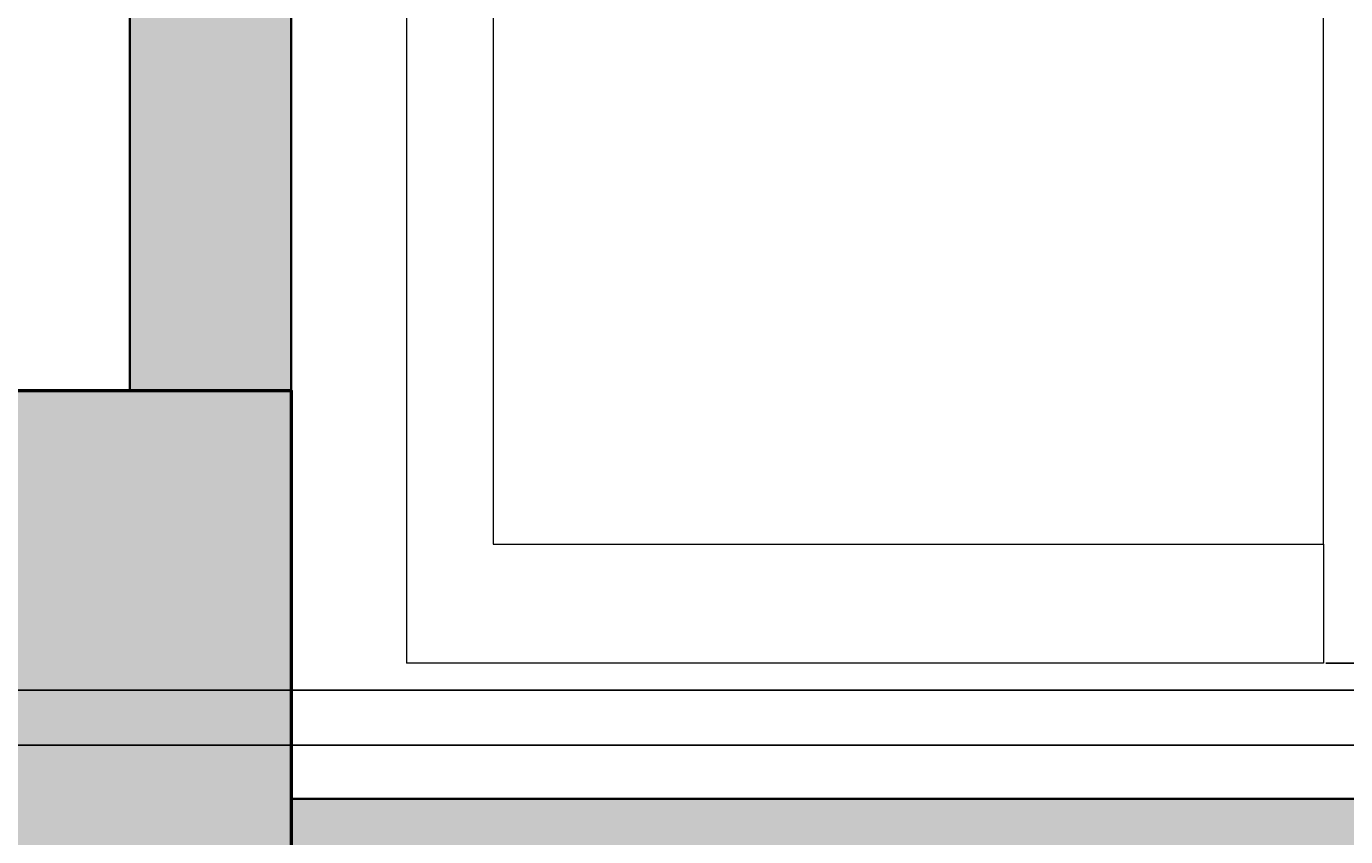
# Model space of a CAD drawing. Units: inches. Extents: x 1998 to 2588, y 1139 to 1977.
# Tile 43 of 134: x 2220 to 2257, y 1592 to 1615. Entities that reach past the tile are written whole.
import ezdxf

# ---------------------------------------------------------------- set-up
doc = ezdxf.new("R2010")
doc.units = ezdxf.units.IN
for name, color, linetype, lineweight in [('A-ANNO-DIMS', 2, 'Continuous', 18), ('A-COLS-PATT', 250, 'Continuous', 13), ('A-WALL-PATT', 252, 'Continuous', 13), ('COLUMN', 10, 'Continuous', 50), ('FUR', 21, 'Continuous', 18), ('WALL', 200, 'Continuous', 35)]:
    doc.layers.add(name, color=color, linetype=linetype, lineweight=lineweight)
doc.styles.get("Standard").update_dxf_attribs({"font": 'arial.ttf'})
doc.dimstyles.get("Standard").update_dxf_attribs({"dimtxt": 0.18, "dimasz": 0.18, "dimexe": 0.18, "dimexo": 0.0625, "dimgap": 0.09, "dimtad": 0, "dimtih": 1, "dimtoh": 1, "dimdec": 4, "dimzin": 0, "dimdsep": 46, "dimtxsty": 'Standard', "dimcen": 0.09, "dimadec": 0, "dimazin": 0, "dimtfac": 1, "dimtdec": 4, "dimtofl": 0, "dimtmove": 0, "dimatfit": 3, "dimfxl": 1, "dimtolj": 1, "dimtzin": 0, "dimarcsym": 0})

# ---------------------------------------------------------------- blocks, each defined once
blk = doc.blocks.new('SOFA-THREE-SEAT')
for p, q in [((71.008, 25.615), (74.336, 25.615)), ((74.336, 25.615), (74.336, 0)), ((0, 0), (74.336, 0))]:
    blk.add_line(p, q)
blk.add_lwpolyline([(3.604, 2.416), (71.008, 2.416), (71.008, 25.615), (3.604, 25.615)], close=True)
blk = doc.blocks.new('*D11')
at = {"layer": 'A-ANNO-DIMS', "color": 0, "lineweight": -2, "transparency": 16777216}
for p, q in [((2256.378, 1671.356), (2267.646, 1671.356)), ((2267.466, 1671.176), (2267.466, 1634.372)), ((2267.466, 1597.201), (2267.466, 1634.005)), ((2256.378, 1597.021), (2267.646, 1597.021))]:
    blk.add_line(p, q, dxfattribs=at)
at = {"layer": 'A-ANNO-DIMS', "color": 0, "transparency": 16777216}
for points in [[(2267.436, 1671.176), (2267.496, 1671.176), (2267.466, 1671.356)], [(2267.436, 1597.201), (2267.496, 1597.201), (2267.466, 1597.021)]]:
    blk.add_solid(points, dxfattribs=at)
at = {"layer": 'Defpoints', "color": 0, "transparency": 16777216}
for p in [(2256.316, 1671.356), (2256.316, 1597.021), (2267.466, 1597.021)]:
    blk.add_point(p, dxfattribs=at)
at = {"layer": 'A-ANNO-DIMS', "color": 0, "transparency": 16777216, "insert": (2267.466, 1634.189), "char_height": 0.18, "attachment_point": 5}
blk.add_mtext('\\A1;SOFA 74 TYP.', dxfattribs=at)
blk = doc.blocks.new('*D30')
at = {"layer": 'A-ANNO-DIMS', "color": 0, "lineweight": -2, "transparency": 16777216}
for p, q in [((2407.91, 1636.732), (1997.843, 1636.732)), ((1998.023, 1636.552), (1998.023, 1615.913)), ((1998.023, 1594.912), (1998.023, 1615.552)), ((2407.91, 1594.732), (1997.843, 1594.732))]:
    blk.add_line(p, q, dxfattribs=at)
at = {"layer": 'A-ANNO-DIMS', "color": 0, "transparency": 16777216}
for points in [[(1997.993, 1636.552), (1998.053, 1636.552), (1998.023, 1636.732)], [(1997.993, 1594.912), (1998.053, 1594.912), (1998.023, 1594.732)]]:
    blk.add_solid(points, dxfattribs=at)
at = {"layer": 'Defpoints', "color": 0, "transparency": 16777216}
for p in [(1998.023, 1636.732), (2407.973, 1636.732), (2407.973, 1594.732)]:
    blk.add_point(p, dxfattribs=at)
at = {"layer": 'A-ANNO-DIMS', "color": 0, "transparency": 16777216, "insert": (1998.023, 1615.732), "char_height": 0.18, "attachment_point": 5}
blk.add_mtext('\\A1;42', dxfattribs=at)
blk = doc.blocks.new('*D34')
at = {"layer": 'A-ANNO-DIMS', "color": 0, "lineweight": -2, "transparency": 16777216}
for p, q in [((2407.91, 1594.732), (1997.843, 1594.732)), ((1998.023, 1594.552), (1998.023, 1558.913)), ((1998.023, 1522.912), (1998.023, 1558.552)), ((2407.91, 1522.732), (1997.843, 1522.732))]:
    blk.add_line(p, q, dxfattribs=at)
at = {"layer": 'A-ANNO-DIMS', "color": 0, "transparency": 16777216}
for points in [[(1997.993, 1594.552), (1998.053, 1594.552), (1998.023, 1594.732)], [(1997.993, 1522.912), (1998.053, 1522.912), (1998.023, 1522.732)]]:
    blk.add_solid(points, dxfattribs=at)
at = {"layer": 'Defpoints', "color": 0, "transparency": 16777216}
for p in [(1998.023, 1594.732), (2407.973, 1594.732), (2407.973, 1522.732)]:
    blk.add_point(p, dxfattribs=at)
at = {"layer": 'A-ANNO-DIMS', "color": 0, "transparency": 16777216, "insert": (1998.023, 1558.732), "char_height": 0.18, "attachment_point": 5}
blk.add_mtext('\\A1;72', dxfattribs=at)
blk = doc.blocks.new('*D39')
at = {"layer": 'A-ANNO-DIMS', "color": 0, "lineweight": -2, "transparency": 16777216}
for p, q in [((2115.035, 1628.742), (2588.309, 1628.742)), ((2588.129, 1628.562), (2588.129, 1612.685)), ((2588.129, 1596.444), (2588.129, 1612.321)), ((2115.035, 1596.264), (2588.309, 1596.264))]:
    blk.add_line(p, q, dxfattribs=at)
at = {"layer": 'A-ANNO-DIMS', "color": 0, "transparency": 16777216}
for points in [[(2588.099, 1628.562), (2588.159, 1628.562), (2588.129, 1628.742)], [(2588.099, 1596.444), (2588.159, 1596.444), (2588.129, 1596.264)]]:
    blk.add_solid(points, dxfattribs=at)
at = {"layer": 'Defpoints', "color": 0, "transparency": 16777216}
for p in [(2114.973, 1628.742), (2588.129, 1628.742), (2114.973, 1596.264)]:
    blk.add_point(p, dxfattribs=at)
at = {"layer": 'A-ANNO-DIMS', "color": 0, "transparency": 16777216, "insert": (2588.129, 1612.503), "char_height": 0.18, "attachment_point": 5}
blk.add_mtext('\\A1;32.48', dxfattribs=at)

msp = doc.modelspace()

# ---------------------------------------------------------------- hatches: boundary and pattern name
at = {"layer": 'A-COLS-PATT'}
h = msp.add_hatch(color=256, dxfattribs=at)
h.dxf.hatch_style = 1
h.paths.add_polyline_path([(2099.4125, 1888.7324), (2087.9729, 1888.7324), (2087.9729, 1868.3278), (2099.4125, 1868.3278)])
h.paths.add_polyline_path([(2234.4125, 1888.7324), (2222.9729, 1888.7324), (2222.9729, 1868.3278), (2234.4125, 1868.3278)])
h.paths.add_polyline_path([(2341.4729, 1886.637), (2330.0332, 1886.637), (2330.0332, 1866.2324), (2341.4729, 1866.2324)])
h.paths.add_polyline_path([(2507.8006, 1882.7324), (2487.396, 1882.7324), (2487.396, 1871.2927), (2507.8006, 1871.2927)])
h.paths.add_polyline_path([(2510.9729, 1766.672), (2490.5682, 1766.672), (2490.5682, 1755.2324), (2510.9729, 1755.2324)])
h.paths.add_polyline_path([(2345.9729, 1759.7324), (2334.5332, 1759.7324), (2334.5332, 1739.3278), (2345.9729, 1739.3278)])
h.paths.add_polyline_path([(2234.4125, 1774.3318), (2222.9729, 1774.3318), (2222.9729, 1753.9272), (2234.4125, 1753.9272)])
h.paths.add_polyline_path([(2099.4125, 1775.637), (2087.9729, 1775.637), (2087.9729, 1755.2324), (2099.4125, 1755.2324)])
h.paths.add_polyline_path([(2098.0956, 1593.7241), (2077.691, 1593.7241), (2077.691, 1582.2845), (2098.0956, 1582.2845)])
h.paths.add_polyline_path([(2227.4729, 1604.637), (2216.0332, 1604.637), (2216.0332, 1584.2324), (2227.4729, 1584.2324)])
h.paths.add_polyline_path([(2345.9729, 1647.5211), (2334.5332, 1647.5211), (2334.5332, 1627.1165), (2345.9729, 1627.1165)])
h.paths.add_polyline_path([(2522.3775, 1641.2324), (2501.9729, 1641.2324), (2501.9729, 1629.7927), (2522.3775, 1629.7927)])
h.paths.add_polyline_path([(2522.3775, 1480.7324), (2501.9729, 1480.7324), (2501.9729, 1469.2927), (2522.3775, 1469.2927)])
h.paths.add_polyline_path([(2345.9729, 1488.5616), (2334.5332, 1488.5616), (2334.5332, 1468.1569), (2345.9729, 1468.1569)])
h.paths.add_polyline_path([(2234.4125, 1486.137), (2227.4729, 1486.137), (2227.4729, 1465.7324), (2234.4125, 1465.7324)])
h.paths.add_polyline_path([(2227.4729, 1486.137), (2222.9729, 1486.137), (2222.9729, 1465.7324), (2227.4729, 1465.7324)])
h.paths.add_polyline_path([(2108.3775, 1470.2324), (2087.9729, 1470.2324), (2087.9729, 1458.7927), (2108.3775, 1458.7927)])
h.paths.add_polyline_path([(2096.9729, 1365.5012), (2087.9729, 1365.5012), (2087.9729, 1345.0966), (2096.9729, 1345.0966)])
h.paths.add_polyline_path([(2087.9729, 1365.5012), (2085.5332, 1365.5012), (2085.5332, 1345.0966), (2087.9729, 1345.0966)])
h.paths.add_polyline_path([(2234.4125, 1285.137), (2222.9729, 1285.137), (2222.9729, 1264.7324), (2234.4125, 1264.7324)])
h.paths.add_polyline_path([(2345.9729, 1285.137), (2334.5332, 1285.137), (2334.5332, 1264.7324), (2345.9729, 1264.7324)])
h.paths.add_polyline_path([(2503.1458, 1240.172), (2482.7412, 1240.172), (2482.7412, 1228.7324), (2503.1458, 1228.7324)])
h.paths.add_polyline_path([(2510.9729, 1369.172), (2490.5682, 1369.172), (2490.5682, 1357.7324), (2510.9729, 1357.7324)])
at = {"layer": 'A-WALL-PATT'}
h = msp.add_hatch(color=256, dxfattribs=at)
h.dxf.hatch_style = 1
h.paths.add_polyline_path([(2222.9729, 1888.7324), (2099.4125, 1888.7324), (2099.4125, 1879.7324), (2222.9729, 1879.7324)])
h.paths.add_polyline_path([(2096.9729, 1868.3278), (2087.9729, 1868.3278), (2087.9729, 1775.637), (2096.9729, 1775.637)])
h.paths.add_polyline_path([(2227.4729, 1868.3278), (2222.9729, 1868.3278), (2222.9729, 1774.3318), (2227.4729, 1774.3318)])
h.paths.add_polyline_path([(2188.3019, 1759.7324), (2138.6074, 1759.7324), (2099.4125, 1759.7324), (2099.4125, 1755.2324), (2176.9729, 1755.2324), (2188.3019, 1755.2324)])
h.paths.add_polyline_path([(2087.9729, 1759.7324), (2059.4729, 1759.7324), (2059.4729, 1702.7324), (2087.9729, 1702.7324), (2087.9729, 1707.2324), (2063.9729, 1707.2324), (2063.9729, 1755.2324), (2087.9729, 1755.2324)])
h.paths.add_polyline_path([(2096.9729, 1755.2324), (2087.9729, 1755.2324), (2087.9729, 1707.2324), (2096.9729, 1707.2324)])
h.paths.add_polyline_path([(2187.0461, 1707.2324), (2105.9729, 1707.2324), (2096.9729, 1707.2324), (2087.9729, 1707.2324), (2087.9729, 1702.7324), (2105.9729, 1702.7324), (2114.9729, 1702.7324), (2187.0461, 1702.7324)])
h.paths.add_polyline_path([(2181.4729, 1719.2028), (2176.9729, 1719.2028), (2176.9729, 1707.2324), (2181.4729, 1707.2324)])
h.paths.add_polyline_path([(2216.0332, 1588.7324), (2114.9729, 1588.7324), (2105.9729, 1588.7324), (2105.9729, 1584.2324), (2216.0332, 1584.2324)])
h.paths.add_polyline_path([(2077.691, 1588.7324), (2061.4729, 1588.7324), (2061.4729, 1584.2324), (2077.691, 1584.2324)])
h.paths.add_polyline_path([(2105.9729, 1588.7324), (2098.0956, 1588.7324), (2098.0956, 1584.2324), (2105.9729, 1584.2324)])
h.paths.add_polyline_path([(2114.9729, 1596.2642), (2110.1012, 1596.2642), (2105.9729, 1596.2642), (2105.9729, 1588.7324), (2114.9729, 1588.7324)])
h.paths.add_polyline_path([(2114.9729, 1584.2324), (2105.9729, 1584.2324), (2105.9729, 1580.249), (2110.1012, 1580.249), (2114.9729, 1580.249)])
h.paths.add_polyline_path([(2114.9729, 1547.7716), (2110.1012, 1547.7716, -0.0318759), (2105.9729, 1548.035), (2105.9729, 1470.2324), (2108.3775, 1470.2324), (2108.3775, 1465.7324), (2186.2943, 1465.7324), (2186.2943, 1470.2324), (2114.9729, 1470.2324)])
h.paths.add_polyline_path([(2227.4729, 1584.2324), (2222.9729, 1584.2324), (2222.9729, 1486.137), (2227.4729, 1486.137)])
h.paths.add_polyline_path([(2295.4138, 1593.2324), (2227.4729, 1593.2324), (2227.4729, 1588.7324), (2295.4138, 1588.7324), (2295.4138, 1591.8729)])
h.paths.add_polyline_path([(2345.9729, 1627.1165), (2341.4729, 1627.1165), (2341.4729, 1593.2324), (2337.2869, 1593.2324), (2337.2869, 1591.8729), (2337.2869, 1588.7324), (2345.9729, 1588.7324)])
h.paths.add_polyline_path([(2291.9729, 1588.7324), (2287.4729, 1588.7324), (2287.4729, 1522.7324), (2291.9729, 1522.7324)])
h.paths.add_polyline_path([(2291.9729, 1522.7324), (2287.4729, 1522.7324), (2227.4729, 1522.7324), (2227.4729, 1518.2324), (2291.9729, 1518.2324)])
h.paths.add_polyline_path([(2295.7347, 1519.5919), (2295.7347, 1522.7324), (2291.9729, 1522.7324), (2291.9729, 1518.2324), (2295.7347, 1518.2324)])
h.paths.add_polyline_path([(2345.9729, 1522.7324), (2337.6078, 1522.7324), (2337.6078, 1519.5919), (2337.6078, 1518.2324), (2341.4729, 1518.2324), (2341.4729, 1488.5616), (2345.9729, 1488.5616)])
h.paths.add_polyline_path([(2345.9729, 1468.1569), (2341.4729, 1468.1569), (2341.4729, 1374.2324), (2227.4729, 1374.2324), (2227.4729, 1369.7324), (2345.9729, 1369.7324)])
h.paths.add_polyline_path([(2345.9729, 1369.7324), (2341.4729, 1369.7324), (2341.4729, 1362.2324), (2345.9729, 1362.2324)])
h.paths.add_polyline_path([(2345.9729, 1317.7324), (2345.9729, 1322.2324), (2341.4729, 1322.2324), (2341.4729, 1285.137), (2345.9729, 1285.137)], flags=17)
h.paths.add_polyline_path([(2356.2096, 1322.2324), (2345.9729, 1322.2324), (2345.9729, 1317.7324), (2356.2096, 1317.7324), (2356.2096, 1319.3088)], flags=17)
h.paths.add_polyline_path([(2393.9729, 1322.2324), (2375.6999, 1322.2324), (2375.6999, 1319.3088, -0.0202458), (2375.636, 1317.7324), (2393.9729, 1317.7324)], flags=17)
h.paths.add_polyline_path([(2398.4729, 1322.2324), (2393.9729, 1322.2324), (2393.9729, 1317.7324), (2393.9729, 1237.7324), (2345.9729, 1237.7324), (2345.9729, 1264.7324), (2341.4729, 1264.7324), (2341.4729, 1228.7324), (2393.9729, 1228.7324), (2482.7412, 1228.7324), (2482.7412, 1237.7324), (2398.4729, 1237.7324), (2398.4729, 1297.1029)])
h.paths.add_polyline_path([(2398.4729, 1362.2324), (2393.9729, 1362.2324), (2393.9729, 1357.7324), (2398.4729, 1357.7324)])
h.paths.add_polyline_path([(2345.9729, 1329.7549), (2341.4729, 1329.7549), (2341.4729, 1322.2324), (2345.9729, 1322.2324)])
h = msp.add_hatch(color=256, dxfattribs=at)
h.dxf.hatch_style = 1
h.paths.add_polyline_path([(2527.4729, 1362.2324), (2510.9729, 1362.2324), (2510.9729, 1357.7324), (2518.4729, 1357.7324), (2518.4729, 1237.7324), (2503.1458, 1237.7324), (2503.1458, 1228.7324), (2527.4729, 1228.7324)])
h.paths.add_polyline_path([(2490.5682, 1362.2324), (2398.4729, 1362.2324), (2398.4729, 1357.7324), (2490.5682, 1357.7324)])
h.paths.add_polyline_path([(2224.9729, 1264.7324), (2222.9729, 1264.7324), (2222.9729, 1232.4125), (2341.4729, 1232.4125), (2341.4729, 1234.4125), (2224.9729, 1234.4125)])
h.paths.add_polyline_path([(2334.5332, 1273.7324), (2264.7638, 1273.7324), (2264.7638, 1269.5611, -0.043659), (2264.3413, 1264.7324), (2334.5332, 1264.7324)])
h.paths.add_polyline_path([(2236.9551, 1273.7324), (2234.4125, 1273.7324), (2234.4125, 1264.7324), (2236.9551, 1264.7324), (2236.9551, 1269.5611)])
h.paths.add_polyline_path([(2222.9729, 1293.2324), (2096.9729, 1293.2324), (2096.9729, 1345.0966), (2087.9729, 1345.0966), (2087.9729, 1284.2324), (2222.9729, 1284.2324), (2222.9729, 1285.137)])
h.paths.add_polyline_path([(2096.9729, 1458.7927), (2087.9729, 1458.7927), (2087.9729, 1417.7324), (2087.9729, 1413.2324), (2096.9729, 1413.2324), (2096.9729, 1417.7324)])
h.paths.add_polyline_path([(2096.9729, 1413.2324), (2087.9729, 1413.2324), (2087.9729, 1365.5012), (2096.9729, 1365.5012), (2096.9729, 1369.3358)])
h.paths.add_polyline_path([(2186.2943, 1417.7324), (2138.6074, 1417.7324), (2096.9729, 1417.7324), (2096.9729, 1413.2324), (2138.6074, 1413.2324), (2186.2943, 1413.2324)])
h.paths.add_polyline_path([(2181.4729, 1465.7324), (2176.9729, 1465.7324), (2176.9729, 1451.6434), (2181.4729, 1451.6434)])
h.paths.add_polyline_path([(2181.4729, 1422.1664), (2176.9729, 1422.1664), (2176.9729, 1417.7324), (2181.4729, 1417.7324)])
h.paths.add_polyline_path([(2063.9729, 1465.7324), (2087.9729, 1465.7324), (2087.9729, 1470.2324), (2059.4729, 1470.2324), (2059.4729, 1413.2324), (2087.9729, 1413.2324), (2087.9729, 1417.7324), (2063.9729, 1417.7324)])
h.paths.add_polyline_path([(2181.4729, 1755.2324), (2176.9729, 1755.2324), (2176.9729, 1748.6798), (2177.0513, 1748.6798), (2181.4729, 1748.6798)])
h.paths.add_polyline_path([(2227.4729, 1707.2324), (2220.4647, 1707.2324), (2220.4647, 1702.7324), (2222.9729, 1702.7324), (2222.9729, 1604.637), (2227.4729, 1604.637)])
h.paths.add_polyline_path([(2114.9729, 1702.7324), (2105.9729, 1702.7324), (2105.9729, 1628.4781, -0.0318759), (2110.1012, 1628.7416), (2114.9729, 1628.7416)])
h.paths.add_polyline_path([(2345.9729, 1739.3278), (2341.4729, 1739.3278), (2341.4729, 1647.5211), (2345.9729, 1647.5211)])
h.paths.add_polyline_path([(2350.6273, 1641.2324), (2345.9729, 1641.2324), (2345.9729, 1636.7324), (2350.6273, 1636.7324), (2350.6273, 1639.8729)])
h.paths.add_polyline_path([(2501.9729, 1641.2324), (2407.9729, 1641.2324), (2392.5005, 1641.2324), (2392.5005, 1639.8729), (2392.5005, 1636.7324), (2501.9729, 1636.7324)])
h.paths.add_polyline_path([(2510.9729, 1755.2324), (2501.9729, 1755.2324), (2501.9729, 1641.2324), (2510.9729, 1641.2324)])
h.paths.add_polyline_path([(2549.1786, 1641.2324), (2522.3775, 1641.2324), (2522.3775, 1636.7324), (2540.1786, 1636.7324), (2540.1786, 1480.7324), (2522.3775, 1480.7324), (2522.3775, 1476.2324), (2549.1786, 1476.2324)])
h.paths.add_polyline_path([(2498.1786, 1594.7324), (2407.9729, 1594.7324), (2407.9729, 1585.7324), (2416.9729, 1585.7324), (2489.1786, 1585.7324), (2489.1786, 1531.7324), (2416.9729, 1531.7324), (2407.9729, 1531.7324), (2407.9729, 1522.7324), (2498.1786, 1522.7324)])
h.paths.add_polyline_path([(2351.6437, 1480.7324), (2345.9729, 1480.7324), (2345.9729, 1476.2324), (2351.6437, 1476.2324), (2351.6437, 1477.5919)])
h.paths.add_polyline_path([(2501.9729, 1480.7324), (2498.1786, 1480.7324), (2407.9729, 1480.7324), (2393.5168, 1480.7324), (2393.5168, 1477.5919), (2393.5168, 1476.2324), (2501.9729, 1476.2324)])

# ---------------------------------------------------------------- linework, layer by layer
at = {"layer": 'COLUMN'}
msp.add_lwpolyline([(2216.0332, 1604.637), (2227.4729, 1604.637), (2227.4729, 1584.2324), (2216.0332, 1584.2324)], close=True, dxfattribs=at)
at = {"layer": 'WALL'}
for p, q in [((2227.4729, 1707.2324), (2227.4729, 1584.2324)), ((2222.9729, 1702.7324), (2222.9729, 1604.637)), ((2296.3298, 1593.2324), (2227.4729, 1593.2324))]:
    msp.add_line(p, q, dxfattribs=at)

# ---------------------------------------------------------------- block references
at = {"layer": 'FUR', "rotation": 270.0000000000001}
msp.add_blockref('SOFA-THREE-SEAT', (2230.701, 1671.3567), dxfattribs=at)

# ---------------------------------------------------------------- dimensions: what is measured, and where the dimension line sits
at = {"layer": 'A-ANNO-DIMS'}
dim = msp.add_linear_dim(base=(2267.4662, 1597.0205), p1=(2256.3158, 1671.3565), p2=(2256.3158, 1597.0205), angle=270, text='SOFA <> TYP.', dimstyle='Standard', override={"dimdec": 0, "dimlfac": 1, "dimrnd": 0, "dimzin": 0, "dimdsep": 46, "dimlunit": 2}, dxfattribs=at)
dim.commit()
dim.dimension.update_dxf_attribs({"geometry": '*D11', "text_midpoint": (2267.4662, 1634.1885)})
for base, p1, p2, override, picture, middle in [((1998.0229, 1636.7324), (2407.9729, 1594.7324), (2407.9729, 1636.7324), {"dimdec": 0, "dimlfac": 1, "dimrnd": 0, "dimzin": 0, "dimdsep": 46, "dimlunit": 2}, '*D30', (1998.0229, 1615.7324)), ((2588.1286, 1628.7416), (2114.9729, 1596.2642), (2114.9729, 1628.7416), {"dimdec": 2, "dimlfac": 1, "dimrnd": 0, "dimzin": 0, "dimdsep": 46, "dimlunit": 2}, '*D39', (2588.1286, 1612.5029)), ((1998.0229, 1594.7324), (2407.9729, 1522.7324), (2407.9729, 1594.7324), {"dimdec": 0, "dimlfac": 1, "dimrnd": 0, "dimzin": 0, "dimdsep": 46, "dimlunit": 2}, '*D34', (1998.0229, 1558.7324))]:
    dim = msp.add_linear_dim(base=base, p1=p1, p2=p2, angle=90, dimstyle='Standard', override=override, dxfattribs=at)
    dim.commit()
    dim.dimension.update_dxf_attribs({"geometry": picture, "text_midpoint": middle})

doc.saveas('drawing.dxf')
